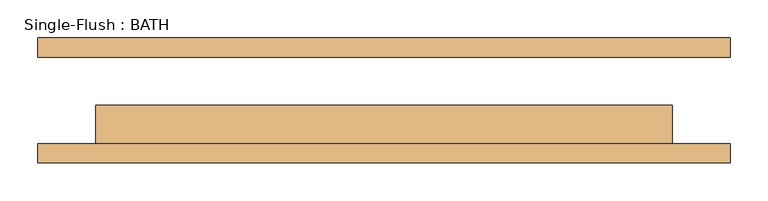
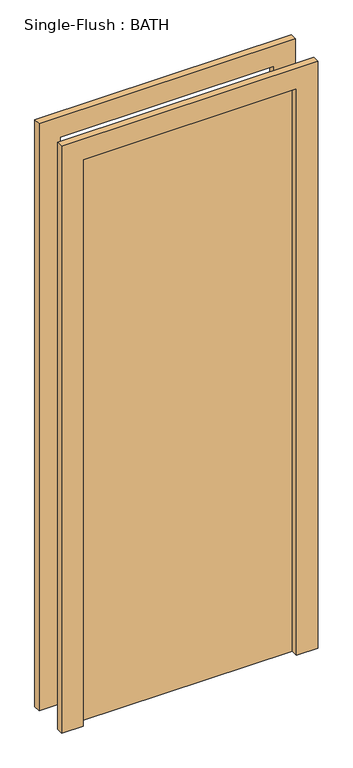
"""IFC4 building model written with IfcOpenShell, lengths in millimetres: door geometry, Single-Flush : BATH."""

from ifc_helpers import new_model, si_unit, frame, origin, origin_with_axes, place, context, project, spatial, polyline, outline, extrude, source, transform, mapped, element, save


def single_flush_bath_78caadf7(model_context):
    return source(origin(), model_context, "Body", "SweptSolid", [
        extrude(outline(polyline([(2209.8, -457.2), (0.0, -457.2), (0.0, -381.0), (2133.6, -381.0), (2133.6, 381.0), (0.0, 381.0), (0.0, 457.2), (2209.8, 457.2), (2209.8, -457.2)])), frame((0.0, -82.55, 0.0), z_axis=(0.0, 1.0, 0.0), x_axis=(0.0, 0.0, 1.0)), (0.0, 0.0, 1.0), 25.4),
        extrude(outline(polyline([(2209.8, 457.2), (2209.8, -457.2), (0.0, -457.2), (0.0, -381.0), (2133.6, -381.0), (2133.6, 381.0), (0.0, 381.0), (0.0, 457.2), (2209.8, 457.2)])), frame((0.0, 57.15, 0.0), z_axis=(0.0, 1.0, 0.0), x_axis=(0.0, 0.0, 1.0)), (0.0, 0.0, 1.0), 25.4),
        extrude(outline(polyline([(381.0, -6.35), (381.0, -57.15), (-381.0, -57.15), (-381.0, -6.35), (381.0, -6.35)])), origin_with_axes(), (0.0, 0.0, 1.0), 2133.6),
    ])


if __name__ == "__main__":
    model = new_model("IFC4")
    model_context = context("Model", 3, world=origin())
    ifc_project = project(units=[si_unit("LENGTHUNIT", "METRE", prefix="MILLI")], contexts=[model_context])
    site = spatial("IfcSite", under=ifc_project)
    building = spatial("IfcBuilding", under=site)
    placement = place(None, origin())
    single_flush_bath_shape = single_flush_bath_78caadf7(model_context)
    element("IfcDoor", 1, ObjectType="Single-Flush : BATH", at=placement, inside=building, context=model_context, shape_type="MappedRepresentation", body=[
        mapped(single_flush_bath_shape, transform((0.0, 0.0, 0.0), x_axis=(1.0, 0.0, 0.0), y_axis=(0.0, 1.0, 0.0), z_axis=(0.0, 0.0, 1.0))),
    ])
    save(model, "model.ifc")

# Revit data of these elements
# Type "Single-Flush : BATH"
#   Type Mark = "9"
#   Construction Type Id = "MDOOR"
#   Assembly Code = "C1020"
#   Analytic Construction = "Metal"
#   Thickness = 0' - 2"
#   Heat Transfer Coefficient (U) = 0.651978 BTU/(h·ft²·°F)
#   Height = 7' - 0"
#   Trim Projection Ext = 0' - 1"
#   Trim Projection Int = 0' - 1"
#   Trim Width = 0' - 3"
#   Width = 2' - 6"
#   Define Thermal Properties by = 1
#   Door Material = Door - Panel
#   Frame Material = Door - Frame
#   Visual Light Transmittance = 0
#   Solar Heat Gain Coefficient = 0
#   Function = (empty or 0)
#   Wall Closure = (empty or 0)
# Element 1 (IfcDoor, "Single-Flush : BATH")
#   Materials on its faces: "Door - Frame", "Door - Panel"
# Materials
#   "Door - Panel": class "Wood", colour RGB 210 159 95, transparency 0, Cost = 0
#   "Door - Frame": colour RGB 118 70 51, transparency 0, Cost = 0
